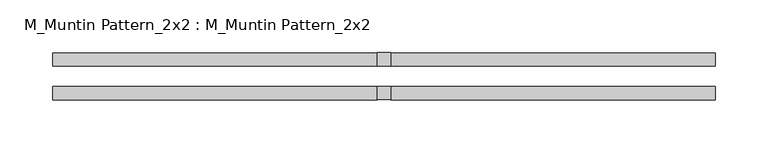
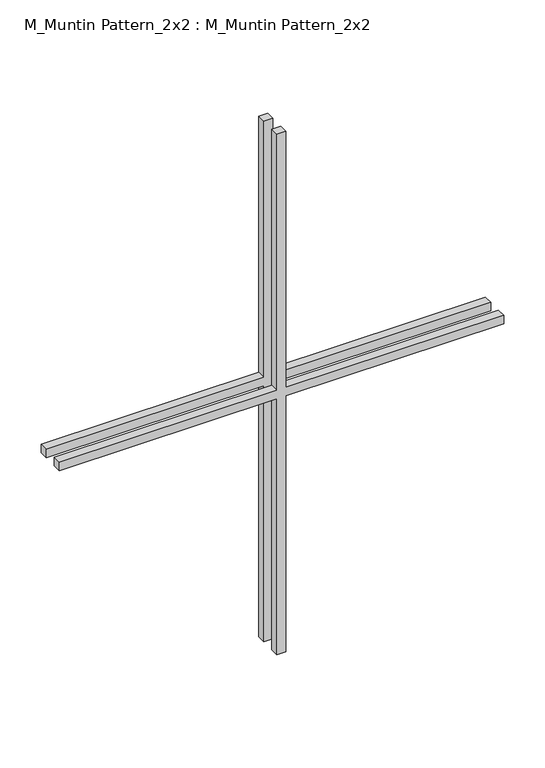
"""IFC4 building model written with IfcOpenShell, lengths in millimetres: proxy geometry, M_Muntin Pattern_2x2 : M_Muntin Pattern_2x2."""

from ifc_helpers import new_model, si_unit, frame, origin, place, context, project, spatial, polyline, outline, extrude, source, transform, mapped, element, save


def m_muntin_pattern_2x2_m_muntin_pattern_2x2_5c2cbe28(model_context):
    return source(origin(), model_context, "Body", "SweptSolid", [
        extrude(outline(polyline([(393.7, -6.35), (393.7, -312.7375), (381.0, -312.7375), (381.0, -6.35), (0.0, -6.35), (0.0, 6.35), (381.0, 6.35), (381.0, 312.7375), (393.7, 312.7375), (393.7, 6.35), (774.7, 6.35), (774.7, -6.35), (393.7, -6.35)])), frame((0.0, -22.225, 0.0), z_axis=(0.0, 1.0, 0.0), x_axis=(0.0, 0.0, 1.0)), (0.0, 0.0, 1.0), 12.7),
        extrude(outline(polyline([(393.7, -6.35), (393.7, -312.7375), (381.0, -312.7375), (381.0, -6.35), (0.0, -6.35), (0.0, 6.35), (381.0, 6.35), (381.0, 312.7375), (393.7, 312.7375), (393.7, 6.35), (774.7, 6.35), (774.7, -6.35), (393.7, -6.35)])), frame((0.0, 9.525, 0.0), z_axis=(0.0, 1.0, 0.0), x_axis=(0.0, 0.0, 1.0)), (0.0, 0.0, 1.0), 12.7),
    ])


if __name__ == "__main__":
    model = new_model("IFC4")
    model_context = context("Model", 3, world=origin())
    ifc_project = project(units=[si_unit("LENGTHUNIT", "METRE", prefix="MILLI")], contexts=[model_context])
    site = spatial("IfcSite", under=ifc_project)
    building = spatial("IfcBuilding", under=site)
    placement = place(None, origin())
    m_muntin_pattern_2x2_m_muntin_pattern_2x2_shape = m_muntin_pattern_2x2_m_muntin_pattern_2x2_5c2cbe28(model_context)
    element("IfcBuildingElementProxy", 1, Name="M_Muntin Pattern_2x2 : M_Muntin Pattern_2x2", ObjectType="M_Muntin Pattern_2x2 : M_Muntin Pattern_2x2", at=placement, inside=building, context=model_context, shape_type="MappedRepresentation", body=[
        mapped(m_muntin_pattern_2x2_m_muntin_pattern_2x2_shape, transform((0.0, 0.0, 0.0), x_axis=(1.0, 0.0, 0.0), y_axis=(0.0, 1.0, 0.0), z_axis=(0.0, 0.0, 1.0))),
    ])
    save(model, "model.ifc")

# Revit data of these elements
# Type "M_Muntin Pattern_2x2 : M_Muntin Pattern_2x2"
#   Width [instance default] = 3' - 11.24409"
#   Thickness = 0' - 0 1/2"
#   Height [instance default] = 3' - 11.24409"
#   Distance = 0' - 0 3/4"
#   Interior Material [instance default] = none
#   Exterior Material [instance default] = none
#   Default Elevation = 0
# Element 1 (IfcBuildingElementProxy, "M_Muntin Pattern_2x2 : M_Muntin Pattern_2x2")
#   Width = 2' - 0 5/8"
#   Height = 2' - 6 1/2"
#   Interior Material = Wood - Stained
#   Exterior Material = Clad - White
#   Materials on its faces: "Clad - White", "Wood - Stained"
# Materials
#   "Clad - White": class "Wood", colour RGB 242 242 238, transparency 0, Cost = 0
#   "Wood - Stained": class "Wood", colour RGB 224 178 126, transparency 0, Cost = 0
